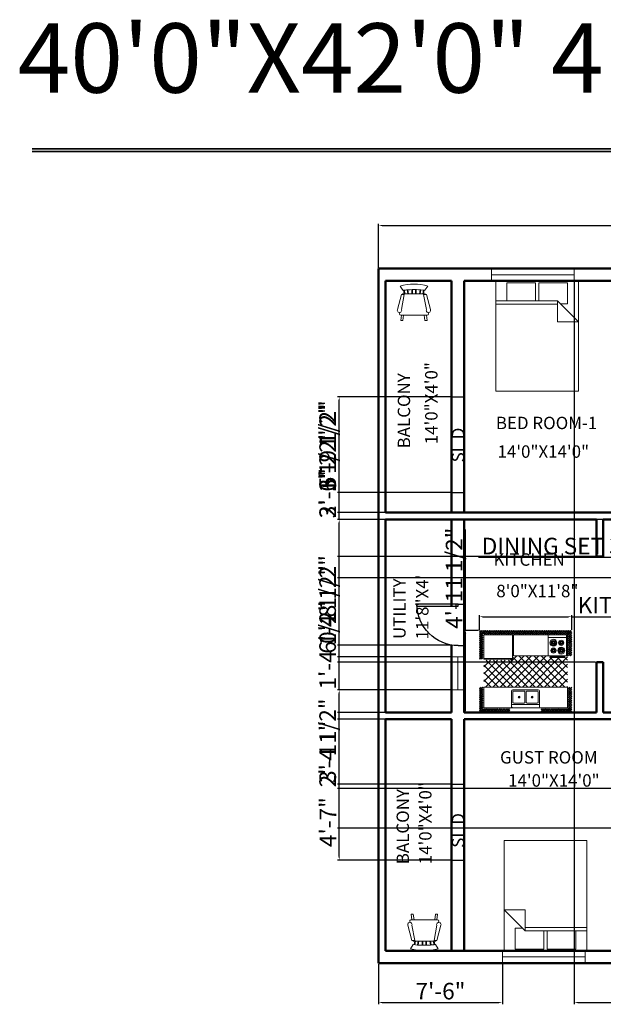
# Model space of a CAD drawing. Units: inches. Extents: x 2744 to 3775, y 2156 to 2963.
# Tile 1 of 4: x 2744 to 3167, y 2223 to 2938. Entities that reach past the tile are written whole.
import ezdxf

# ---------------------------------------------------------------- set-up
doc = ezdxf.new("R2010")
doc.units = ezdxf.units.IN
for name, color, linetype, lineweight in [('A-ANNO-DIMS', 2, 'Continuous', 18), ('A-ANNO-TEXT', 7, 'Continuous', 18), ('A-ANNO-TTLB', 210, 'Continuous', 35), ('A-AREA-IDEN', 7, 'Continuous', 25), ('A-DOOR', 3, 'Continuous', 25), ('A-FLOR-FIXT', 9, 'Continuous', 18), ('A-FURN', 8, 'Continuous', 18), ('A-GLAZ', 4, 'Continuous', 18), ('A-WALL', 7, 'Continuous', 50)]:
    doc.layers.add(name, color=color, linetype=linetype, lineweight=lineweight)
doc.styles.get("Standard").update_dxf_attribs({"font": 'arial.ttf'})
doc.dimstyles.new('ISO-25', dxfattribs={"dimtxt": 12, "dimasz": 2.5, "dimexe": 1.25, "dimexo": 0.625, "dimtad": 1, "dimdec": 1, "dimlunit": 4, "dimtxsty": 'Standard', "dimcen": 2.5, "dimadec": 0, "dimazin": 0, "dimtfac": 1, "dimtdec": 1, "dimtmove": 0, "dimatfit": 3, "dimfxl": 1, "dimarcsym": 0})

# ---------------------------------------------------------------- blocks, each defined once
blk = doc.blocks.new('Bed - Queen')
for p, q in [((0, -80.00003), (0, 0)), ((0, 0), (59.99999, 0)), ((59.99999, 0), (59.99999, -80.00003)), ((7.99999, -1.2), (28.79998, -1.2)), ((7.99999, -14.4), (7.99999, -1.2)), ((28.79998, -1.2), (28.79998, -14.4)), ((31.19999, -1.2), (51.99999, -1.2)), ((31.19999, -14.4), (31.19999, -1.2)), ((51.99999, -1.2), (51.99999, -16.4)), ((0, -14.4), (44.8, -14.4)), ((44.8, -16.8), (0, -16.8)), ((59.99999, -29.6), (44.8, -14.4)), ((44.8, -14.4), (44.8, -29.6)), ((51.99999, -16.4), (46.79936, -16.4)), ((44.8, -29.6), (59.99999, -29.6)), ((59.99999, -80.00003), (0, -80.00003))]:
    blk.add_line(p, q)
blk = doc.blocks.new('Kitchen Layout - 7 x 8 ft')
for p, q in [((-5, 81.3), (2.7, 89)), ((-5, 83.4), (0.6, 89)), ((-5, 85.6), (-1.6, 89)), ((-5, 87.7), (-3.7, 89)), ((-1, 85), (-5, 89)), ((-1, 82.9), (-5, 86.9)), ((-1, 80.7), (-5, 84.7)), ((-5, 79.2), (-1, 83.2)), ((-1, 78.6), (-5, 82.6)), ((-5, 77.1), (-1, 81.1)), ((-1, 76.5), (-5, 80.5)), ((1.1, 85), (-2.9, 89)), ((3.2, 85), (-0.8, 89)), ((0.8, 85), (4.8, 89)), ((5.3, 85), (1.3, 89)), ((2.9, 85), (6.9, 89)), ((7.5, 85), (3.5, 89)), ((5, 85), (9, 89)), ((9.6, 85), (5.6, 89)), ((7.2, 85), (11.2, 89)), ((11.7, 85), (7.7, 89)), ((9.3, 85), (13.3, 89)), ((13.8, 85), (9.8, 89)), ((11.4, 85), (15.4, 89)), ((15.9, 85), (11.9, 89)), ((13.5, 85), (17.5, 89)), ((18.1, 85), (14.1, 89)), ((15.7, 85), (19.7, 89)), ((20.2, 85), (16.2, 89)), ((17.8, 85), (21.8, 89)), ((22.3, 85), (18.3, 89)), ((19.9, 85), (23.9, 89)), ((24.4, 85), (20.4, 89)), ((22, 85), (26, 89)), ((26.5, 85), (22.5, 89)), ((24.1, 85), (28.1, 89)), ((28.7, 85), (24.7, 89)), ((26.3, 85), (30.3, 89)), ((30.8, 85), (26.8, 89)), ((28.4, 85), (32.4, 89)), ((32.9, 85), (28.9, 89)), ((30.5, 85), (34.5, 89)), ((35, 85), (31, 89)), ((32.6, 85), (36.6, 89)), ((37.2, 85), (33.2, 89)), ((34, 84), (96, 84)), ((34, 60), (34, 84)), ((34.7, 85), (38.7, 89)), ((39.3, 85), (35.3, 89)), ((36.9, 85), (40.9, 89)), ((41.4, 85), (37.4, 89)), ((39, 85), (43, 89)), ((43.5, 85), (39.5, 89)), ((41.1, 85), (45.1, 89)), ((45.6, 85), (41.6, 89)), ((43.2, 85), (47.2, 89)), ((47.8, 85), (43.8, 89)), ((45.4, 85), (49.4, 89)), ((49.9, 85), (45.9, 89)), ((47.5, 85), (51.5, 89)), ((52, 85), (48, 89)), ((49.6, 85), (53.6, 89)), ((54.1, 85), (50.1, 89)), ((51.7, 85), (55.7, 89)), ((56.2, 85), (52.2, 89)), ((53.8, 85), (57.8, 89)), ((58.4, 85), (54.4, 89)), ((56, 85), (60, 89)), ((60.5, 85), (56.5, 89)), ((58.1, 85), (62.1, 89)), ((62.6, 85), (58.6, 89)), ((60.2, 85), (64.2, 89)), ((64.7, 85), (60.7, 89)), ((62.3, 85), (66.3, 89)), ((66.9, 85), (62.9, 89)), ((64.4, 85), (68.4, 89)), ((69, 85), (65, 89)), ((66.6, 85), (70.6, 89)), ((71.1, 85), (67.1, 89)), ((68.7, 85), (72.7, 89)), ((73.2, 85), (69.2, 89)), ((70.8, 85), (74.8, 89)), ((75.3, 85), (71.3, 89)), ((72.9, 85), (76.9, 89)), ((77.5, 85), (73.5, 89)), ((74, 81), (95, 81)), ((75.1, 85), (79.1, 89)), ((79.6, 85), (75.6, 89)), ((77.2, 85), (81.2, 89)), ((81.7, 85), (77.7, 89)), ((79.3, 85), (83.3, 89)), ((83.8, 85), (79.8, 89)), ((81.4, 85), (85.4, 89)), ((85.9, 85), (81.9, 89)), ((83.5, 85), (87.5, 89)), ((88.1, 85), (84.1, 89)), ((85.7, 85), (89.7, 89)), ((90.2, 85), (86.2, 89)), ((87.8, 85), (91.8, 89)), ((92.3, 85), (88.3, 89)), ((89.9, 85), (93.9, 89)), ((94.4, 85), (90.4, 89)), ((92, 85), (96, 89)), ((96.6, 85), (92.6, 89)), ((94.1, 85), (98.1, 89)), ((101, 82.7), (94.7, 89)), ((96, 84), (96, 60)), ((96.3, 85), (100.3, 89)), ((101, 84.8), (96.8, 89)), ((97, 83.6), (101, 87.6)), ((97, 81.5), (101, 85.5)), ((101, 80.6), (97, 84.6)), ((97, 79.4), (101, 83.4)), ((101, 78.4), (97, 82.4)), ((97, 77.2), (101, 81.2)), ((101, 76.3), (97, 80.3)), ((101, 86.9), (98.9, 89)), ((-5, 75), (-1, 79)), ((-1, 74.4), (-5, 78.4)), ((-5, 72.8), (-1, 76.8)), ((-1, 72.2), (-5, 76.2)), ((-5, 70.7), (-1, 74.7)), ((-1, 70.1), (-5, 74.1)), ((-5, 68.6), (-1, 72.6)), ((-1, 68), (-5, 72)), ((-5, 66.5), (-1, 70.5)), ((-1, 65.9), (-5, 69.9)), ((-5, 64.3), (-1, 68.3)), ((97, 75.1), (101, 79.1)), ((101, 74.2), (97, 78.2)), ((97, 73), (101, 77)), ((101, 72.1), (97, 76.1)), ((97, 70.9), (101, 74.9)), ((101, 69.9), (97, 73.9)), ((97, 68.8), (101, 72.8)), ((101, 67.8), (97, 71.8)), ((97, 66.6), (101, 70.6)), ((101, 65.7), (97, 69.7)), ((97, 64.5), (101, 68.5)), ((-1, 63.8), (-5, 67.8)), ((-5, 62.2), (-1, 66.2)), ((-1, 61.6), (-5, 65.6)), ((-5, 60.1), (-1, 64.1)), ((-1, 59.5), (-5, 63.5)), ((-5, 58), (-1, 62)), ((-1, 57.4), (-5, 61.4)), ((-1.7, 56), (-5, 59.3)), ((-3.8, 56), (-5, 57.2)), ((-4.9, 56), (-1, 59.9)), ((-2.7, 56), (-1, 57.7)), ((0, 57), (33, 57)), ((10.4, 24), (45.9, 59.5)), ((18.9, 24), (54.4, 59.5)), ((27.4, 24), (62.9, 59.5)), ((33, 55.1), (37.4, 59.5)), ((67.7, 24), (33.7, 58)), ((96, 60), (34, 60)), ((35.9, 24), (71.4, 59.5)), ((76.2, 24), (40.7, 59.5)), ((44.3, 24), (77.8, 57.5)), ((84.7, 24), (49.2, 59.5)), ((52.8, 24), (86.3, 57.5)), ((93.2, 24), (57.7, 59.5)), ((61.3, 24), (96, 58.7)), ((96, 29.7), (66.2, 59.5)), ((96, 38.1), (76.6, 57.5)), ((80, 60), (80, 59)), ((82, 59), (82, 60)), ((96, 46.6), (85.1, 57.5)), ((87, 59), (87, 60)), ((89, 60), (89, 59)), ((96, 55.1), (93.6, 57.5)), ((101, 63.6), (97, 67.6)), ((97, 62.4), (101, 66.4)), ((101, 61.5), (97, 65.5)), ((97, 60.3), (101, 64.3)), ((100.3, 60), (97, 63.3)), ((98.2, 60), (97, 61.2)), ((98.8, 60), (101, 62.2)), ((101, 60), (101, 60)), ((0, 30.6), (24.4, 55)), ((0, 39.1), (15.9, 55)), ((0, 47.5), (7.5, 55)), ((25.3, 24), (0, 49.3)), ((1.9, 24), (32.9, 55)), ((33.8, 24), (2.8, 55)), ((42.3, 24), (11.3, 55)), ((50.7, 24), (19.7, 55)), ((59.2, 24), (28.2, 55)), ((31, 55), (31, 56)), ((32, 55), (31, 55)), ((32, 56), (32, 55)), ((69.8, 24), (96, 50.2)), ((16.8, 24), (0, 40.8)), ((78.3, 24), (96, 41.7)), ((-5, 21.9), (-2.9, 24)), ((-5, 19.8), (-1, 23.8)), ((-1, 19.2), (-5, 23.2)), ((-1, 21.3), (-3.7, 24)), ((-1, 23.5), (-1.5, 24)), ((8.3, 24), (0, 32.3)), ((0, 24), (96, 24)), ((0, 0), (0, 24)), ((86.8, 24), (96, 33.2)), ((95.2, 24), (96, 24.8)), ((96, 24), (96, 0)), ((97, 22.1), (98.9, 24)), ((97, 20), (101, 24)), ((101, 19), (97, 23)), ((101, 21.2), (98.2, 24)), ((101, 23.3), (100.3, 24)), ((-5, 17.7), (-1, 21.7)), ((-1, 17.1), (-5, 21.1)), ((-5, 15.6), (-1, 19.6)), ((-1, 15), (-5, 19)), ((-5, 13.4), (-1, 17.4)), ((-1, 12.8), (-5, 16.8)), ((-5, 11.3), (-1, 15.3)), ((-1, 10.7), (-5, 14.7)), ((-5, 9.2), (-1, 13.2)), ((-1, 8.6), (-5, 12.6)), ((47.3, 6.5), (47.3, 18.5)), ((48.8, 18.5), (48.8, 6.5)), ((97, 17.9), (101, 21.9)), ((101, 16.9), (97, 20.9)), ((97, 15.7), (101, 19.7)), ((101, 14.8), (97, 18.8)), ((97, 13.6), (101, 17.6)), ((101, 12.7), (97, 16.7)), ((97, 11.5), (101, 15.5)), ((101, 10.5), (97, 14.5)), ((97, 9.4), (101, 13.4)), ((101, 8.4), (97, 12.4)), ((-5, 7.1), (-1, 11.1)), ((-1, 6.5), (-5, 10.5)), ((-5, 4.9), (-1, 8.9)), ((-1, 4.4), (-5, 8.4)), ((-5, 2.8), (-1, 6.8)), ((-1, 2.2), (-5, 6.2)), ((-5, 0.7), (-1, 4.7)), ((-1, 0.1), (-5, 4.1)), ((-5, -1.4), (-1, 2.6)), ((2, -5), (-5, 2)), ((-5, -3.5), (-1, 0.5)), ((96, 0), (0, 0)), ((64, 4), (32, 4)), ((93.2, -5), (101, 2.8)), ((95.4, -5), (101, 0.6)), ((97, 7.2), (101, 11.2)), ((101, 6.3), (97, 10.3)), ((97, 5.1), (101, 9.1)), ((101, 4.2), (97, 8.2)), ((97, 3), (101, 7)), ((101, 2.1), (97, 6.1)), ((97, 0.9), (101, 4.9)), ((101, -0.1), (97, 3.9)), ((101, -2.2), (97, 1.8)), ((-0.1, -5), (-5, -0.1)), ((-2.2, -5), (-5, -2.2)), ((-4.4, -5), (-5, -4.4)), ((-4.3, -5), (-0.3, -1)), ((-2.2, -5), (1.8, -1)), ((-0.1, -5), (3.9, -1)), ((4.1, -5), (0.1, -1)), ((2, -5), (6, -1)), ((6.2, -5), (2.2, -1)), ((4.1, -5), (8.1, -1)), ((8.4, -5), (4.4, -1)), ((6.3, -5), (10.3, -1)), ((10.5, -5), (6.5, -1)), ((8.4, -5), (12.4, -1)), ((12.6, -5), (8.6, -1)), ((10.5, -5), (14.5, -1)), ((14.7, -5), (10.7, -1)), ((12.6, -5), (16.6, -1)), ((16.8, -5), (12.8, -1)), ((14.8, -5), (18.8, -1)), ((19, -5), (15, -1)), ((16.9, -5), (20.9, -1)), ((21.1, -5), (17.1, -1)), ((19, -5), (23, -1)), ((23.2, -5), (19.2, -1)), ((21.1, -5), (25.1, -1)), ((25.3, -5), (21.3, -1)), ((23.2, -5), (27.2, -1)), ((27.5, -5), (23.5, -1)), ((25.4, -5), (29.4, -1)), ((29.6, -5), (25.6, -1)), ((27.5, -5), (30, -2.5)), ((30, -3.3), (27.7, -1)), ((29.6, -5), (30, -4.6)), ((30, -1.2), (29.8, -1)), ((66, -2.5), (67.5, -1)), ((66, -4.7), (69.7, -1)), ((69.9, -5), (66, -1.1)), ((67.8, -5), (66, -3.2)), ((67.8, -5), (71.8, -1)), ((72, -5), (68, -1)), ((69.9, -5), (73.9, -1)), ((74.1, -5), (70.1, -1)), ((72, -5), (76, -1)), ((76.2, -5), (72.2, -1)), ((74.1, -5), (78.1, -1)), ((78.4, -5), (74.4, -1)), ((76.3, -5), (80.3, -1)), ((80.5, -5), (76.5, -1)), ((78.4, -5), (82.4, -1)), ((82.6, -5), (78.6, -1)), ((80.5, -5), (84.5, -1)), ((84.7, -5), (80.7, -1)), ((82.6, -5), (86.6, -1)), ((86.9, -5), (82.9, -1)), ((84.8, -5), (88.8, -1)), ((89, -5), (85, -1)), ((86.9, -5), (90.9, -1)), ((91.1, -5), (87.1, -1)), ((89, -5), (93, -1)), ((93.2, -5), (89.2, -1)), ((91.1, -5), (95.1, -1)), ((95.3, -5), (91.3, -1)), ((97.5, -5), (93.5, -1)), ((99.6, -5), (95.6, -1)), ((101, -4.3), (97, -0.3)), ((97.5, -5), (101, -1.5)), ((99.6, -5), (101, -3.6))]:
    blk.add_line(p, q)
for points in [[(0, 56), (0, 84), (33, 84), (33, 56)], [(74, 60), (74, 84), (95, 84), (95, 60)], [(76, 58), (76, 59), (93, 59), (93, 58)]]:
    blk.add_lwpolyline(points, close=True)
for points in [[(32, 1.5), (32, 19.5)], [(33.5, 21), (62.5, 21)], [(33.5, 6.5), (33.5, 18.5)], [(34.5, 19.5), (46.3, 19.5)], [(49.8, 19.5), (61.5, 19.5)], [(62.5, 18.5), (62.5, 6.5)], [(64, 19.5), (64, 1.5)], [(62.5, 0), (33.5, 0)], [(46.3, 5.5), (34.5, 5.5)], [(61.5, 5.5), (49.8, 5.5)]]:
    blk.add_lwpolyline(points)
for centre, radius in [((80, 75), 4), ((80, 75), 3), ((80, 66), 3), ((80, 75), 2), ((80, 66), 2), ((80, 75), 1), ((89, 66), 4), ((89, 75), 3), ((89, 66), 3), ((89, 75), 2), ((89, 66), 2), ((89, 75), 1), ((80, 66), 1), ((89, 66), 1), ((40.5, 12.5), 1), ((40.5, 12.5), 0.5), ((55.5, 12.5), 1), ((55.5, 12.5), 0.5)]:
    blk.add_circle(centre, radius)
for centre, radius, start, end in [((33.5, 19.5), 1.5, 90, 180), ((34.5, 18.5), 1, 90, 180), ((46.3, 18.5), 1, 0, 90), ((49.8, 18.5), 1, 90, 180), ((61.5, 18.5), 1, 0, 90), ((62.5, 19.5), 1.5, 0, 90), ((33.5, 1.5), 1.5, 180, 270), ((34.5, 6.5), 1, 180, 270), ((46.3, 6.5), 1, 270, 0), ((49.8, 6.5), 1, 180, 270), ((61.5, 6.5), 1, 270, 0), ((62.5, 1.5), 1.5, 270, 0)]:
    blk.add_arc(centre, radius, start, end)
blk = doc.blocks.new('Chair - Rocking')
for p, q in [((-8, -4.5), (-10, -1.5)), ((-8.23428, -6.99939), (-8.3093, -7.47958)), ((-8.23041, -7), (8.23915, -7)), ((-7.5, -4.5), (-7, -7)), ((-6.5, -7), (-7.02225, -4.43)), ((-4.5, -7), (-4.96674, -4.19951)), ((-4, -7), (-4.40532, -4.16272)), ((-1.5, -4.05012), (-1.5, -7)), ((-1, -7), (-1, -4.05012)), ((1, -7), (1, -4.04655)), ((1.5, -4.05012), (1.5, -7)), ((4, -7), (4.40187, -4.18694)), ((4.5, -7), (4.96761, -4.19437)), ((6.5, -7), (7, -4.4057)), ((7.5, -4.5), (7, -7)), ((8, -4.5), (10, -1.5)), ((8.31071, -7.48854), (8.23449, -7.00073)), ((-9, -7.5), (-12, -18.49999)), ((-7, -7.5), (-9, -7.5)), ((-9, -18.49999), (-7, -7.5)), ((7, -7.5), (9, -7.5)), ((9, -18.49999), (7, -7.5)), ((9, -7.5), (12, -18.49999)), ((-10.36644, -20.64523), (-10.5, -21.49999)), ((10.5, -21.49999), (10.3575, -20.58798)), ((-9, -22.49999), (-9.5, -26.49999)), ((0, -22.49999), (-9.5, -22.49999)), ((-9.5, -26.49999), (-8, -26.49999)), ((-8, -26.49999), (-7.5, -22.49999)), ((0, -22.49999), (9.5, -22.49999)), ((8, -26.49999), (7.5, -22.49999)), ((9.5, -26.49999), (8, -26.49999)), ((9, -22.49999), (9.5, -26.49999))]:
    blk.add_line(p, q)
for centre, radius, start, end in [((0, -34.08333), 34.08333, 72.93847, 107.0615), ((0, -68.25004), 64.25, 93.92211, 97.15267), ((0, -68.25004), 64.25, 82.84733, 93.92211), ((-10.5, -18.99999), 1.58114, 161.5651, 18.43495), ((10.5, -18.99999), 1.58114, 161.5651, 18.43495), ((-9.5, -21.49999), 1, 180, 270), ((9.5, -21.49999), 1, 270, 0)]:
    blk.add_arc(centre, radius, start, end)
blk = doc.blocks.new('*U2')
for p, q in [((0, 0), (0, -6)), ((40, 0), (40, -6))]:
    blk.add_line(p, q)
blk.add_lwpolyline([(0, 0), (0, 40), (1.75, 40), (1.75, 0)], close=True)
blk.add_arc((0, 0), 40, 0, 90)
blk = doc.blocks.new('*D14')
at = {"layer": 'A-ANNO-DIMS', "color": 0, "lineweight": -2, "transparency": 16777216}
for p, q in [((3003.92, 2757.73), (3003.92, 2789.67)), ((3006.42, 2788.42), (3481.42, 2788.42)), ((3483.92, 2757.73), (3483.92, 2789.67))]:
    blk.add_line(p, q, dxfattribs=at)
at = {"layer": 'A-ANNO-DIMS', "color": 0, "transparency": 16777216}
for points in [[(3006.42, 2788.84), (3006.42, 2788), (3003.92, 2788.42)], [(3481.42, 2788.84), (3481.42, 2788), (3483.92, 2788.42)]]:
    blk.add_solid(points, dxfattribs=at)
at = {"layer": 'Defpoints', "color": 0, "transparency": 16777216}
for p in [(3483.92, 2788.42), (3003.92, 2757.1), (3483.92, 2757.1)]:
    blk.add_point(p, dxfattribs=at)
at = {"layer": 'A-ANNO-DIMS', "color": 0, "transparency": 16777216, "insert": (3243.92, 2795.17), "char_height": 12, "attachment_point": 5}
blk.add_mtext("40'", dxfattribs=at)
blk = doc.blocks.new('WIN-60IN')
blk.add_line((0, 4.5), (60, 4.5))
blk.add_lwpolyline([(0, 9), (60, 9), (60, 0), (0, 0)], close=True)
blk = doc.blocks.new('WIN-24IN')
blk.add_line((0, 4.5), (24, 4.5))
blk.add_lwpolyline([(0, 9), (24, 9), (24, 0), (0, 0)], close=True)
blk = doc.blocks.new('*D30')
at = {"layer": 'A-ANNO-DIMS', "color": 0, "lineweight": -2, "transparency": 16777216}
for p, q in [((3077.09, 2495.06), (3077.09, 2505.72)), ((3079.59, 2504.47), (3141.49, 2504.47)), ((3143.99, 2495.06), (3143.99, 2505.72)), ((3143.99, 2504.47), (3301.12, 2504.47))]:
    blk.add_line(p, q, dxfattribs=at)
at = {"layer": 'A-ANNO-DIMS', "color": 0, "transparency": 16777216}
for points in [[(3079.59, 2504.89), (3079.59, 2504.06), (3077.09, 2504.47)], [(3141.49, 2504.89), (3141.49, 2504.06), (3143.99, 2504.47)]]:
    blk.add_solid(points, dxfattribs=at)
at = {"layer": 'Defpoints', "color": 0, "transparency": 16777216}
for p in [(3143.99, 2504.47), (3077.09, 2494.44), (3143.99, 2494.44)]:
    blk.add_point(p, dxfattribs=at)
at = {"layer": 'A-ANNO-DIMS', "color": 0, "transparency": 16777216, "insert": (3223.81, 2511.3), "char_height": 12, "attachment_point": 5}
blk.add_mtext('KITCHEN UNIT 5\'-7"', dxfattribs=at)
blk = doc.blocks.new('*D31')
at = {"layer": 'A-ANNO-DIMS', "color": 0, "lineweight": -2, "transparency": 16777216}
for p, q in [((3067.05, 2494.44), (3067.05, 2567.86)), ((3076.46, 2494.44), (3065.8, 2494.44)), ((3067.05, 2437.6), (3067.05, 2491.94)), ((3076.46, 2435.1), (3065.8, 2435.1))]:
    blk.add_line(p, q, dxfattribs=at)
at = {"layer": 'A-ANNO-DIMS', "color": 0, "transparency": 16777216}
for points in [[(3066.63, 2491.94), (3067.47, 2491.94), (3067.05, 2494.44)], [(3066.63, 2437.6), (3067.47, 2437.6), (3067.05, 2435.1)]]:
    blk.add_solid(points, dxfattribs=at)
at = {"layer": 'Defpoints', "color": 0, "transparency": 16777216}
for p in [(3067.05, 2494.44), (3077.09, 2494.44), (3077.09, 2435.1)]:
    blk.add_point(p, dxfattribs=at)
at = {"layer": 'A-ANNO-DIMS', "color": 0, "transparency": 16777216, "insert": (3060.22, 2532.4), "char_height": 12, "attachment_point": 5, "rotation": 90}
blk.add_mtext('4\'-11 1/2"', dxfattribs=at)
blk = doc.blocks.new('*D32')
at = {"layer": 'A-ANNO-DIMS', "color": 0, "lineweight": -2, "transparency": 16777216}
for p, q in [((3212.07, 2547.39), (3076.42, 2547.39)), ((3212.07, 2541.68), (3212.07, 2548.64)), ((3251.79, 2547.39), (3214.57, 2547.39)), ((3254.29, 2541.68), (3254.29, 2548.64))]:
    blk.add_line(p, q, dxfattribs=at)
at = {"layer": 'A-ANNO-DIMS', "color": 0, "transparency": 16777216}
for points in [[(3214.57, 2547.81), (3214.57, 2546.97), (3212.07, 2547.39)], [(3251.79, 2547.81), (3251.79, 2546.97), (3254.29, 2547.39)]]:
    blk.add_solid(points, dxfattribs=at)
at = {"layer": 'Defpoints', "color": 0, "transparency": 16777216}
for p in [(3212.07, 2547.39), (3212.07, 2541.06), (3254.29, 2541.06)]:
    blk.add_point(p, dxfattribs=at)
at = {"layer": 'A-ANNO-DIMS', "color": 0, "transparency": 16777216, "insert": (3143, 2554.22), "char_height": 12, "attachment_point": 5}
blk.add_mtext('DINING SET 3\'-6"', dxfattribs=at)
blk = doc.blocks.new('*D34')
at = {"layer": 'A-ANNO-DIMS', "color": 0, "lineweight": -2, "transparency": 16777216}
for p, q in [((3145.86, 2747.48), (3145.86, 2223.25)), ((3174.92, 2747.48), (3174.92, 2223.25)), ((3148.36, 2224.5), (3172.42, 2224.5)), ((3174.92, 2224.5), (3210.78, 2224.5))]:
    blk.add_line(p, q, dxfattribs=at)
at = {"layer": 'A-ANNO-DIMS', "color": 0, "transparency": 16777216}
for points in [[(3148.36, 2224.92), (3148.36, 2224.09), (3145.86, 2224.5)], [(3172.42, 2224.92), (3172.42, 2224.09), (3174.92, 2224.5)]]:
    blk.add_solid(points, dxfattribs=at)
at = {"layer": 'Defpoints', "color": 0, "transparency": 16777216}
for p in [(3145.86, 2748.1), (3174.92, 2748.1), (3174.92, 2224.5)]:
    blk.add_point(p, dxfattribs=at)
at = {"layer": 'A-ANNO-DIMS', "color": 0, "transparency": 16777216, "insert": (3194.1, 2231.26), "char_height": 12, "attachment_point": 5}
blk.add_mtext('2\'-5"', dxfattribs=at)
blk = doc.blocks.new('*D38')
at = {"layer": 'A-ANNO-DIMS', "color": 0, "lineweight": -2, "transparency": 16777216}
for p, q in [((3003.92, 2252.48), (3003.92, 2223.25)), ((3093.68, 2252.48), (3093.68, 2223.25)), ((3006.42, 2224.5), (3091.18, 2224.5))]:
    blk.add_line(p, q, dxfattribs=at)
at = {"layer": 'A-ANNO-DIMS', "color": 0, "transparency": 16777216}
for points in [[(3006.42, 2224.92), (3006.42, 2224.09), (3003.92, 2224.5)], [(3091.18, 2224.92), (3091.18, 2224.09), (3093.68, 2224.5)]]:
    blk.add_solid(points, dxfattribs=at)
at = {"layer": 'Defpoints', "color": 0, "transparency": 16777216}
for p in [(3003.92, 2253.1), (3093.68, 2253.1), (3093.68, 2224.5)]:
    blk.add_point(p, dxfattribs=at)
at = {"layer": 'A-ANNO-DIMS', "color": 0, "transparency": 16777216, "insert": (3048.8, 2231.26), "char_height": 12, "attachment_point": 5}
blk.add_mtext('7\'-6"', dxfattribs=at)
blk = doc.blocks.new('*D48')
at = {"layer": 'A-ANNO-DIMS', "color": 0, "lineweight": -2, "transparency": 16777216}
for p, q in [((3056.3, 2664.1), (2974.07, 2664.1)), ((2975.32, 2597.03), (2975.32, 2661.6)), ((3056.3, 2594.53), (2974.07, 2594.53))]:
    blk.add_line(p, q, dxfattribs=at)
at = {"layer": 'A-ANNO-DIMS', "color": 0, "transparency": 16777216}
for points in [[(2974.91, 2661.6), (2975.74, 2661.6), (2975.32, 2664.1)], [(2974.91, 2597.03), (2975.74, 2597.03), (2975.32, 2594.53)]]:
    blk.add_solid(points, dxfattribs=at)
at = {"layer": 'Defpoints', "color": 0, "transparency": 16777216}
for p in [(2975.32, 2664.1), (3056.92, 2664.1), (3056.92, 2594.53)]:
    blk.add_point(p, dxfattribs=at)
at = {"layer": 'A-ANNO-DIMS', "color": 0, "transparency": 16777216, "insert": (2968.49, 2629.32), "char_height": 12, "attachment_point": 5, "rotation": 90}
blk.add_mtext('5\'-9 1/2"', dxfattribs=at)
blk = doc.blocks.new('*D50')
at = {"layer": 'A-ANNO-DIMS', "color": 0, "lineweight": -2, "transparency": 16777216}
for p, q in [((3056.3, 2382.98), (2974.07, 2382.98)), ((2975.32, 2330.41), (2975.32, 2380.48)), ((3056.3, 2327.91), (2974.07, 2327.91))]:
    blk.add_line(p, q, dxfattribs=at)
at = {"layer": 'A-ANNO-DIMS', "color": 0, "transparency": 16777216}
for points in [[(2974.91, 2380.48), (2975.74, 2380.48), (2975.32, 2382.98)], [(2974.91, 2330.41), (2975.74, 2330.41), (2975.32, 2327.91)]]:
    blk.add_solid(points, dxfattribs=at)
at = {"layer": 'Defpoints', "color": 0, "transparency": 16777216}
for p in [(2975.32, 2382.98), (3056.92, 2382.98), (3056.92, 2327.91)]:
    blk.add_point(p, dxfattribs=at)
at = {"layer": 'A-ANNO-DIMS', "color": 0, "transparency": 16777216, "insert": (2968.7, 2355.45), "char_height": 12, "attachment_point": 5, "rotation": 90}
blk.add_mtext('4\'-7"', dxfattribs=at)
blk = doc.blocks.new('*D51')
at = {"layer": 'A-ANNO-DIMS', "color": 0, "lineweight": -2, "transparency": 16777216}
for p, q in [((3161.3, 2548.26), (2974.07, 2548.26)), ((2975.32, 2474.02), (2975.32, 2545.76)), ((3161.3, 2471.52), (2974.07, 2471.52))]:
    blk.add_line(p, q, dxfattribs=at)
at = {"layer": 'A-ANNO-DIMS', "color": 0, "transparency": 16777216}
for points in [[(2974.91, 2545.76), (2975.74, 2545.76), (2975.32, 2548.26)], [(2974.91, 2474.02), (2975.74, 2474.02), (2975.32, 2471.52)]]:
    blk.add_solid(points, dxfattribs=at)
at = {"layer": 'Defpoints', "color": 0, "transparency": 16777216}
for p in [(2975.32, 2548.26), (3161.92, 2548.26), (3161.92, 2471.52)]:
    blk.add_point(p, dxfattribs=at)
at = {"layer": 'A-ANNO-DIMS', "color": 0, "transparency": 16777216, "insert": (2968.49, 2509.89), "char_height": 12, "attachment_point": 5, "rotation": 90}
blk.add_mtext('6\'-4 1/2"', dxfattribs=at)
blk = doc.blocks.new('*D53')
at = {"layer": 'A-ANNO-DIMS', "color": 0, "lineweight": -2, "transparency": 16777216}
for p, q in [((2975.32, 2575.1), (2975.32, 2638.71)), ((3325.3, 2575.1), (2974.07, 2575.1)), ((2975.32, 2535.1), (2975.32, 2572.6)), ((3325.3, 2532.6), (2974.07, 2532.6))]:
    blk.add_line(p, q, dxfattribs=at)
at = {"layer": 'A-ANNO-DIMS', "color": 0, "transparency": 16777216}
for points in [[(2974.91, 2572.6), (2975.74, 2572.6), (2975.32, 2575.1)], [(2974.91, 2535.1), (2975.74, 2535.1), (2975.32, 2532.6)]]:
    blk.add_solid(points, dxfattribs=at)
at = {"layer": 'Defpoints', "color": 0, "transparency": 16777216}
for p in [(2975.32, 2575.1), (3325.92, 2575.1), (3325.92, 2532.6)]:
    blk.add_point(p, dxfattribs=at)
at = {"layer": 'A-ANNO-DIMS', "color": 0, "transparency": 16777216, "insert": (2968.49, 2608.16), "char_height": 12, "attachment_point": 5, "rotation": 90}
blk.add_mtext('3\'-6 1/2"', dxfattribs=at)
blk = doc.blocks.new('*D54')
at = {"layer": 'A-ANNO-DIMS', "color": 0, "lineweight": -2, "transparency": 16777216}
for p, q in [((2975.32, 2379.79), (2975.32, 2443.61)), ((3233.3, 2379.79), (2974.07, 2379.79)), ((2975.32, 2353.6), (2975.32, 2377.29)), ((3233.3, 2351.1), (2974.07, 2351.1))]:
    blk.add_line(p, q, dxfattribs=at)
at = {"layer": 'A-ANNO-DIMS', "color": 0, "transparency": 16777216}
for points in [[(2974.91, 2377.29), (2975.74, 2377.29), (2975.32, 2379.79)], [(2974.91, 2353.6), (2975.74, 2353.6), (2975.32, 2351.1)]]:
    blk.add_solid(points, dxfattribs=at)
at = {"layer": 'Defpoints', "color": 0, "transparency": 16777216}
for p in [(2975.32, 2379.79), (3233.92, 2379.79), (3233.92, 2351.1)]:
    blk.add_point(p, dxfattribs=at)
at = {"layer": 'A-ANNO-DIMS', "color": 0, "transparency": 16777216, "insert": (2968.49, 2412.95), "char_height": 12, "attachment_point": 5, "rotation": 90}
blk.add_mtext('2\'-4 1/2"', dxfattribs=at)
blk = doc.blocks.new('*D55')
at = {"layer": 'A-ANNO-DIMS', "color": 0, "lineweight": -2, "transparency": 16777216}
for p, q in [((2975.32, 2451.39), (2975.32, 2513.87)), ((3056.3, 2451.39), (2974.07, 2451.39)), ((2975.32, 2437.6), (2975.32, 2448.89)), ((3056.3, 2435.1), (2974.07, 2435.1))]:
    blk.add_line(p, q, dxfattribs=at)
at = {"layer": 'A-ANNO-DIMS', "color": 0, "transparency": 16777216}
for points in [[(2974.91, 2448.89), (2975.74, 2448.89), (2975.32, 2451.39)], [(2974.91, 2437.6), (2975.74, 2437.6), (2975.32, 2435.1)]]:
    blk.add_solid(points, dxfattribs=at)
at = {"layer": 'Defpoints', "color": 0, "transparency": 16777216}
for p in [(2975.32, 2451.39), (3056.92, 2451.39), (3056.92, 2435.1)]:
    blk.add_point(p, dxfattribs=at)
at = {"layer": 'A-ANNO-DIMS', "color": 0, "transparency": 16777216, "insert": (2968.49, 2483.88), "char_height": 12, "attachment_point": 5, "rotation": 90}
blk.add_mtext('1\'-4 1/2"', dxfattribs=at)
blk = doc.blocks.new('*D56')
at = {"layer": 'A-ANNO-DIMS', "color": 0, "lineweight": -2, "transparency": 16777216}
for p, q in [((2975.32, 2483.94), (2975.32, 2547.55)), ((3056.3, 2483.94), (2974.07, 2483.94)), ((2975.32, 2477.89), (2975.32, 2481.44)), ((3056.3, 2475.39), (2974.07, 2475.39))]:
    blk.add_line(p, q, dxfattribs=at)
at = {"layer": 'A-ANNO-DIMS', "color": 0, "transparency": 16777216}
for points in [[(2974.91, 2481.44), (2975.74, 2481.44), (2975.32, 2483.94)], [(2974.91, 2477.89), (2975.74, 2477.89), (2975.32, 2475.39)]]:
    blk.add_solid(points, dxfattribs=at)
at = {"layer": 'Defpoints', "color": 0, "transparency": 16777216}
for p in [(2975.32, 2483.94), (3056.92, 2483.94), (3056.92, 2475.39)]:
    blk.add_point(p, dxfattribs=at)
at = {"layer": 'A-ANNO-DIMS', "color": 0, "transparency": 16777216, "insert": (2968.49, 2517), "char_height": 12, "attachment_point": 5, "rotation": 90}
blk.add_mtext('0\'-8 1/2"', dxfattribs=at)
blk = doc.blocks.new('*D60')
at = {"layer": 'A-ANNO-DIMS', "color": 0, "lineweight": -2, "transparency": 16777216}
for p, q in [((2975.32, 2594.53), (2975.32, 2657.02)), ((3056.3, 2594.53), (2974.07, 2594.53)), ((2975.32, 2582.6), (2975.32, 2592.03)), ((3056.3, 2580.1), (2974.07, 2580.1))]:
    blk.add_line(p, q, dxfattribs=at)
at = {"layer": 'A-ANNO-DIMS', "color": 0, "transparency": 16777216}
for points in [[(2974.91, 2592.03), (2975.74, 2592.03), (2975.32, 2594.53)], [(2974.91, 2582.6), (2975.74, 2582.6), (2975.32, 2580.1)]]:
    blk.add_solid(points, dxfattribs=at)
at = {"layer": 'Defpoints', "color": 0, "transparency": 16777216}
for p in [(2975.32, 2594.53), (3056.92, 2594.53), (3056.92, 2580.1)]:
    blk.add_point(p, dxfattribs=at)
at = {"layer": 'A-ANNO-DIMS', "color": 0, "transparency": 16777216, "insert": (2968.49, 2627.03), "char_height": 12, "attachment_point": 5, "rotation": 90}
blk.add_mtext('1\'-2 1/2"', dxfattribs=at)
blk = doc.blocks.new('*D62')
at = {"layer": 'A-ANNO-DIMS', "color": 0, "lineweight": -2, "transparency": 16777216}
for p, q in [((3056.3, 2430.1), (2974.07, 2430.1)), ((2975.32, 2385.48), (2975.32, 2427.6)), ((3056.3, 2382.98), (2974.07, 2382.98))]:
    blk.add_line(p, q, dxfattribs=at)
at = {"layer": 'A-ANNO-DIMS', "color": 0, "transparency": 16777216}
for points in [[(2974.91, 2427.6), (2975.74, 2427.6), (2975.32, 2430.1)], [(2974.91, 2385.48), (2975.74, 2385.48), (2975.32, 2382.98)]]:
    blk.add_solid(points, dxfattribs=at)
at = {"layer": 'Defpoints', "color": 0, "transparency": 16777216}
for p in [(2975.32, 2430.1), (3056.92, 2430.1), (3056.92, 2382.98)]:
    blk.add_point(p, dxfattribs=at)
at = {"layer": 'A-ANNO-DIMS', "color": 0, "transparency": 16777216, "insert": (2968.57, 2406.54), "char_height": 12, "attachment_point": 5, "rotation": 90}
blk.add_mtext('3\'-11"', dxfattribs=at)
blk = doc.blocks.new('*D63')
at = {"layer": 'A-ANNO-DIMS', "color": 0, "lineweight": -2, "transparency": 16777216}
for p, q in [((2975.32, 2575.1), (2975.32, 2610.96)), ((3161.3, 2575.1), (2974.07, 2575.1)), ((2975.32, 2550.76), (2975.32, 2572.6)), ((3161.3, 2548.26), (2974.07, 2548.26))]:
    blk.add_line(p, q, dxfattribs=at)
at = {"layer": 'A-ANNO-DIMS', "color": 0, "transparency": 16777216}
for points in [[(2974.91, 2572.6), (2975.74, 2572.6), (2975.32, 2575.1)], [(2974.91, 2550.76), (2975.74, 2550.76), (2975.32, 2548.26)]]:
    blk.add_solid(points, dxfattribs=at)
at = {"layer": 'Defpoints', "color": 0, "transparency": 16777216}
for p in [(2975.32, 2575.1), (3161.92, 2575.1), (3161.92, 2548.26)]:
    blk.add_point(p, dxfattribs=at)
at = {"layer": 'A-ANNO-DIMS', "color": 0, "transparency": 16777216, "insert": (2968.57, 2594.28), "char_height": 12, "attachment_point": 5, "rotation": 90}
blk.add_mtext('2\'-3"', dxfattribs=at)

msp = doc.modelspace()

# ---------------------------------------------------------------- linework, layer by layer
at = {"layer": 'A-ANNO-TTLB'}
for p, q in [((2752.61, 2844.08), (3775.35, 2844.08)), ((2752.61, 2842.08), (3775.35, 2842.08))]:
    msp.add_line(p, q, dxfattribs=at)
at = {"layer": 'A-DOOR'}
for p, q in [((3056.92, 2664.1), (3065.92, 2664.1)), ((3056.92, 2594.53), (3065.92, 2594.53)), ((3056.92, 2382.98), (3065.92, 2382.98)), ((3056.92, 2327.91), (3065.92, 2327.91))]:
    msp.add_line(p, q, dxfattribs=at)
at = {"layer": 'A-WALL'}
for p, q in [((3003.92, 2757.1), (3483.92, 2757.1)), ((3003.92, 2253.1), (3003.92, 2757.1)), ((3008.92, 2748.1), (3056.92, 2748.1)), ((3008.92, 2580.1), (3008.92, 2748.1)), ((3012.92, 2748.1), (3056.92, 2748.1)), ((3056.92, 2580.1), (3056.92, 2748.1)), ((3065.92, 2748.1), (3174.92, 2748.1)), ((3065.92, 2580.1), (3065.92, 2748.1)), ((3065.92, 2748.1), (3174.92, 2748.1)), ((3008.92, 2580.1), (3065.92, 2580.1)), ((3065.92, 2580.1), (3190.29, 2580.1)), ((3008.92, 2575.1), (3065.92, 2575.1)), ((3008.92, 2435.1), (3008.92, 2575.1)), ((3056.92, 2512.24), (3056.92, 2575.1)), ((3065.92, 2575.1), (3161.92, 2575.1)), ((3065.92, 2435.1), (3065.92, 2575.1)), ((3161.92, 2548.26), (3161.92, 2575.1)), ((3166.92, 2575.1), (3325.92, 2575.1)), ((3166.92, 2548.26), (3166.92, 2575.1)), ((3161.92, 2548.26), (3166.92, 2548.26)), ((3056.92, 2435.1), (3056.92, 2483.94)), ((3161.92, 2435.1), (3161.92, 2471.52)), ((3161.92, 2471.52), (3166.92, 2471.52)), ((3166.92, 2435.1), (3166.92, 2471.52)), ((3056.92, 2435.1), (3008.92, 2435.1)), ((3056.92, 2430.1), (3008.92, 2430.1)), ((3008.92, 2262.1), (3008.92, 2430.1)), ((3056.92, 2262.1), (3056.92, 2430.1)), ((3161.92, 2435.1), (3065.92, 2435.1)), ((3065.92, 2262.1), (3065.92, 2430.1)), ((3233.92, 2430.1), (3065.92, 2430.1)), ((3238.92, 2435.1), (3166.92, 2435.1)), ((3065.92, 2262.1), (3008.92, 2262.1)), ((3174.92, 2262.1), (3065.92, 2262.1)), ((3483.92, 2253.1), (3003.92, 2253.1))]:
    msp.add_line(p, q, dxfattribs=at)

# ---------------------------------------------------------------- block references
at = {"layer": 'A-DOOR', "xscale": -0.75, "yscale": 0.75, "zscale": 0.75, "rotation": 90}
msp.add_blockref('*U2', (3061.75, 2513.55), dxfattribs=at)
at = {"layer": 'A-FLOR-FIXT', "xscale": 0.6312038519867083, "yscale": 0.6312038519867083, "zscale": 0.6312038519867083}
msp.add_blockref('Kitchen Layout - 7 x 8 ft', (3080.24, 2438.26), dxfattribs=at)
at = {"layer": 'A-FURN'}
for name, p in [('Chair - Rocking', (3029.57, 2745.85)), ('Bed - Queen', (3088.92, 2748.04))]:
    msp.add_blockref(name, p, dxfattribs=at)
at = {"layer": 'A-FURN', "rotation": 180}
for name, p in [('Bed - Queen', (3155.04, 2262.1)), ('Chair - Rocking', (3037.11, 2262.1))]:
    msp.add_blockref(name, p, dxfattribs=at)
at = {"layer": 'A-GLAZ'}
for p in [(3085.86, 2748.1), (3093.68, 2253.1)]:
    msp.add_blockref('WIN-60IN', p, dxfattribs=at)
at = {"layer": 'A-GLAZ', "rotation": 90.00000000000043}
msp.add_blockref('WIN-24IN', (3065.92, 2451.39), dxfattribs=at)

# ---------------------------------------------------------------- texts
at = {"layer": 'A-ANNO-TEXT'}
for p in [(3066.08, 2616.51), (3066.08, 2336.84)]:
    msp.add_text('SL D', height=9, rotation=90, dxfattribs=at).set_placement(p)
at = {"layer": 'A-ANNO-TTLB'}
msp.add_text('40\'0"X42\'0" 4BHK HOUSE PLAN', height=50.3636, dxfattribs=at).set_placement((2742.18, 2884.73))
at = {"layer": 'A-AREA-IDEN'}
for s, p in [('14\'0"X4\'0"', (3046.66, 2629.65)), ('BALCONY', (3026.8, 2626.63)), ('UTILITY', (3023.5, 2488.32)), ('11\'8"X4\'', (3040.09, 2488.03)), ('BALCONY', (3025.96, 2324.9)), ('14\'0"X4\'0"', (3042.31, 2324.9))]:
    msp.add_text(s, height=9, rotation=90, dxfattribs=at).set_placement(p)
for s, p in [('BED ROOM-1', (3088.98, 2640.59)), ('14\'0"X14\'0"', (3090.21, 2619.83)), ('KITCHEN', (3087.28, 2541.48)), ('8\'0"X11\'8"', (3089.29, 2518.66)), ('GUST ROOM', (3092.03, 2397.94)), ('14\'0"X14\'0"', (3097.87, 2381.18))]:
    msp.add_text(s, height=9, dxfattribs=at).set_placement(p)

# ---------------------------------------------------------------- dimensions: what is measured, and where the dimension line sits
at = {"layer": 'A-ANNO-DIMS'}
for base, p1, p2, override, picture, middle in [((3483.92, 2788.42), (3003.92, 2757.1), (3483.92, 2757.1), {"dimclrd": 0, "dimclre": 0, "dimclrt": 0}, '*D14', (3243.92, 2795.17)), ((3174.92, 2224.5), (3145.86, 2748.1), (3174.92, 2748.1), {"dimdec": 1, "dimlfac": 1, "dimrnd": 0, "dimzin": 1, "dimdsep": 46, "dimlunit": 4, "dimfrac": 2}, '*D34', (3194.1, 2231.26)), ((3093.68, 2224.5), (3003.92, 2253.1), (3093.68, 2253.1), {"dimdec": 1, "dimlfac": 1, "dimrnd": 0, "dimzin": 1, "dimdsep": 46, "dimlunit": 4, "dimfrac": 2}, '*D38', (3048.8, 2231.26))]:
    dim = msp.add_linear_dim(base=base, p1=p1, p2=p2, dimstyle='ISO-25', override=override, dxfattribs=at)
    dim.commit()
    dim.dimension.update_dxf_attribs({"geometry": picture, "text_midpoint": middle})
for base, p1, p2, picture, middle in [((2975.32, 2664.1), (3056.92, 2594.53), (3056.92, 2664.1), '*D48', (2968.49, 2629.32)), ((2975.32, 2594.53), (3056.92, 2580.1), (3056.92, 2594.53), '*D60', (2968.49, 2627.03)), ((2975.32, 2575.1), (3325.92, 2532.6), (3325.92, 2575.1), '*D53', (2968.49, 2608.16)), ((2975.32, 2575.1), (3161.92, 2548.26), (3161.92, 2575.1), '*D63', (2968.57, 2594.28)), ((3067.05, 2494.44), (3077.09, 2435.1), (3077.09, 2494.44), '*D31', (3060.22, 2532.4)), ((2975.32, 2548.26), (3161.92, 2471.52), (3161.92, 2548.26), '*D51', (2968.49, 2509.89)), ((2975.3224, 2483.9418), (3056.9224, 2475.3863), (3056.9224, 2483.9418), '*D56', (2968.4928, 2516.9973)), ((2975.32, 2451.39), (3056.92, 2435.1), (3056.92, 2451.39), '*D55', (2968.49, 2483.88)), ((2975.32, 2379.79), (3233.92, 2351.1), (3233.92, 2379.79), '*D54', (2968.49, 2412.95)), ((2975.32, 2430.1), (3056.92, 2382.98), (3056.92, 2430.1), '*D62', (2968.57, 2406.54)), ((2975.32, 2382.98), (3056.92, 2327.91), (3056.92, 2382.98), '*D50', (2968.7, 2355.45))]:
    dim = msp.add_linear_dim(base=base, p1=p1, p2=p2, angle=90, dimstyle='ISO-25', override={"dimdec": 1, "dimlfac": 1, "dimrnd": 0, "dimzin": 1, "dimdsep": 46, "dimlunit": 4, "dimfrac": 2}, dxfattribs=at)
    dim.commit()
    dim.dimension.update_dxf_attribs({"geometry": picture, "text_midpoint": middle})
dim = msp.add_linear_dim(base=(3212.07, 2547.39), p1=(3254.29, 2541.06), p2=(3212.07, 2541.06), angle=180, text='DINING SET <>', dimstyle='ISO-25', override={"dimdec": 1, "dimlfac": 1, "dimrnd": 0, "dimzin": 1, "dimdsep": 46, "dimlunit": 4, "dimfrac": 2}, dxfattribs=at)
dim.commit()
dim.dimension.update_dxf_attribs({"geometry": '*D32', "text_midpoint": (3143, 2554.22)})
dim = msp.add_linear_dim(base=(3143.99, 2504.47), p1=(3077.09, 2494.44), p2=(3143.99, 2494.44), text='KITCHEN UNIT <>', dimstyle='ISO-25', override={"dimdec": 1, "dimlfac": 1, "dimrnd": 0, "dimzin": 1, "dimdsep": 46, "dimlunit": 4, "dimfrac": 2}, dxfattribs=at)
dim.commit()
dim.dimension.update_dxf_attribs({"geometry": '*D30', "text_midpoint": (3223.81, 2511.3)})

doc.saveas('drawing.dxf')
